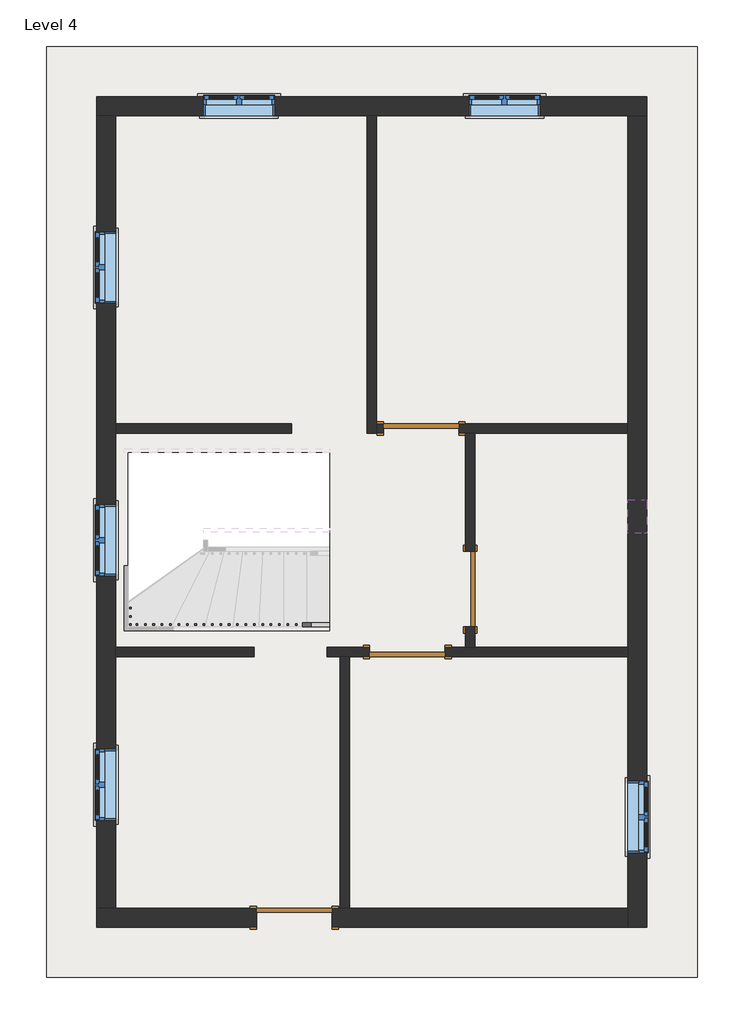
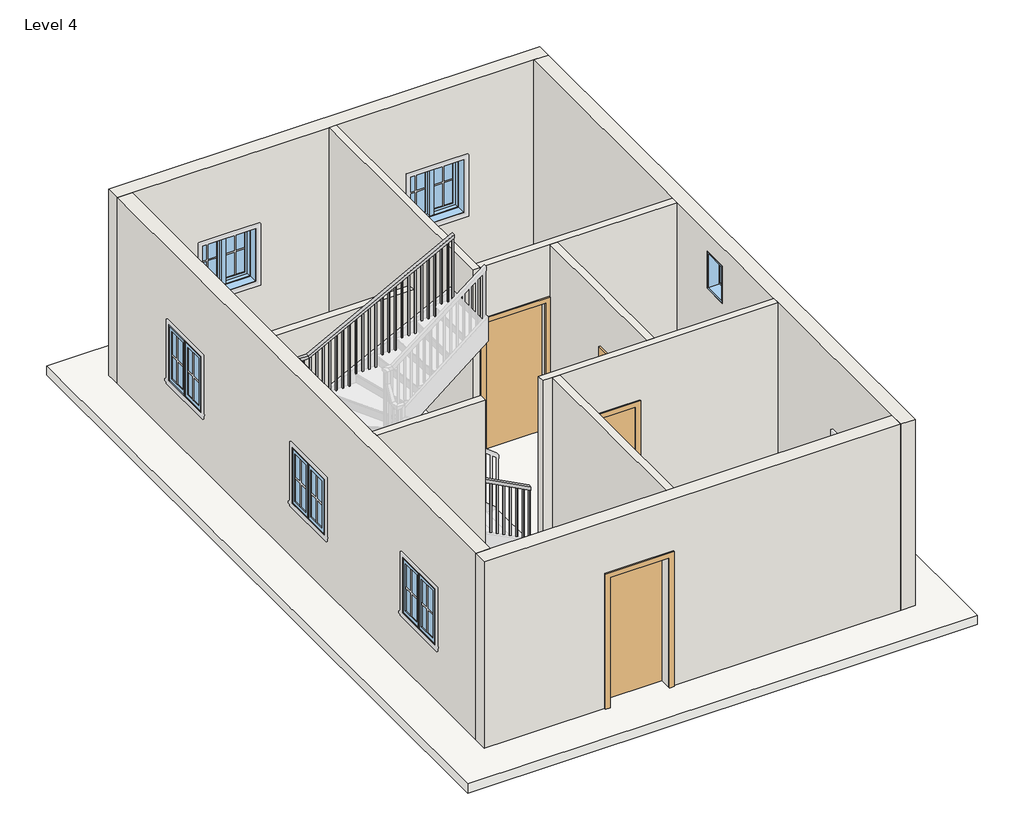
# One storey, part 1 of 2: 11 walls, 7 windows, 4 doors, 1 railing, 1 roof.
"""IFC4 building model written with IfcOpenShell, lengths in millimetres."""

from ifc_helpers import new_model, si_unit, frame, origin, place, context, project, spatial, polyline, outline, extrude, faceted_brep, transform, mapped, element, save
from components import door_e5f9f3c4, door_305aa2a5, door_a90ba1ad, window_aa618e30, window_339605e1

model = new_model("IFC4")

# Units and contexts
model_context = context("Model", 3, world=origin())
ifc_project = project(units=[si_unit("LENGTHUNIT", "METRE", prefix="MILLI")], contexts=[model_context])

# Site, building, storey
site = spatial("IfcSite", under=ifc_project)
building = spatial("IfcBuilding", under=site)
storey = spatial("IfcBuildingStorey", under=building, Name="Level 4", Elevation=6400.8)

# Doors
placement = place(None, origin())
door_shape = door_e5f9f3c4(model_context)
element("IfcDoor", 1, ObjectType="Single-Flush : 36\" x 84\"", at=placement, inside=storey, context=model_context, shape_type="MappedRepresentation", body=[
    mapped(door_shape, transform((-78.9949167, -802.9070853, 6400.8), x_axis=(0.0, -1.0, 0.0), y_axis=(1.0, 0.0, 0.0), z_axis=(0.0, 0.0, 1.0))),
])
element("IfcDoor", 2, ObjectType="Single-Flush : 36\" x 84\"", at=placement, inside=storey, context=model_context, shape_type="MappedRepresentation", body=[
    mapped(door_shape, transform((-840.9949167, -1564.9070853, 6400.8), x_axis=(-1.0, 0.0, 0.0), y_axis=(0.0, -1.0, 0.0), z_axis=(0.0, 0.0, 1.0))),
])
door_2_shape = door_305aa2a5(model_context)
element("IfcDoor", 3, ObjectType="Single-Flush : 36\" x 84\"", at=placement, inside=storey, context=model_context, shape_type="MappedRepresentation", body=[
    mapped(door_2_shape, transform((-675.8949167, 1140.1929147, 6400.8), x_axis=(-1.0, 0.0, 0.0), y_axis=(0.0, -1.0, 0.0), z_axis=(0.0, 0.0, 1.0))),
])
door_3_shape = door_a90ba1ad(model_context)
element("IfcDoor", 4, ObjectType="Single-Flush : 36\" x 84\"", at=placement, inside=storey, context=model_context, shape_type="MappedRepresentation", body=[
    mapped(door_3_shape, transform((-2212.5949167, -4784.3570853, 6400.8), x_axis=(-1.0, 0.0, 0.0), y_axis=(0.0, -1.0, 0.0), z_axis=(0.0, 0.0, 1.0))),
])

# Railing
element("IfcRailing", 5, ObjectType="Handrail - Rectangular", at=placement, inside=storey, context=model_context, shape_type="SolidModel", body=[
    faceted_brep([(-1783.4132248, -1260.1070853, 7484.5333333), (-1783.4132248, -1260.1070853, 7427.0742652), (-1783.4132248, -1209.3070853, 7427.0742652), (-1783.4132248, -1209.3070853, 7484.5333333), (-4041.1382869, -1260.1070853, 8677.8239201), (-4053.7373514, -1260.1070853, 8627.0239201), (-4053.7373514, -1209.3070853, 8627.0239201), (-4041.1382869, -1209.3070853, 8677.8239201), (-4225.5449167, -1260.1070853, 8677.8239201), (-4225.5449167, -1260.1070853, 8627.0239201), (-4174.7449167, -1209.3070853, 8627.0239201), (-4174.7449167, -1209.3070853, 8677.8239201), (-4225.5449167, -972.7952032, 8677.8239201), (-4225.5449167, -964.8446271, 8627.0239201), (-4174.7449167, -964.8446271, 8627.0239201), (-4174.7449167, -972.7952032, 8677.8239201), (-4225.5449167, 560.7810325, 9169.9094132), (-4225.5449167, 568.7316087, 9119.1094132), (-4174.7449167, 568.7316087, 9119.1094132), (-4174.7449167, 560.7810325, 9169.9094132), (-4225.5449167, 848.0929147, 9169.9094132), (-4225.5449167, 848.0929147, 9119.1094132), (-4174.7449167, 797.2929147, 9119.1094132), (-4174.7449167, 797.2929147, 9169.9094132), (-4041.1382869, 848.0929147, 9169.9094132), (-4028.5392223, 848.0929147, 9119.1094132), (-4028.5392223, 797.2929147, 9119.1094132), (-4041.1382869, 797.2929147, 9169.9094132), (-1783.4132248, 848.0929147, 10363.2), (-1783.4132248, 797.2929147, 10363.2), (-1783.4132248, 797.2929147, 10305.7409318), (-1783.4132248, 848.0929147, 10305.7409318)], [[[0, 1, 2, 3]], [[1, 0, 4, 5]], [[2, 1, 5, 6]], [[3, 2, 6, 7]], [[0, 3, 7, 4]], [[5, 4, 8, 9]], [[6, 5, 9, 10]], [[7, 6, 10, 11]], [[4, 7, 11, 8]], [[9, 8, 12, 13]], [[10, 9, 13, 14]], [[11, 10, 14, 15]], [[8, 11, 15, 12]], [[13, 12, 16, 17]], [[14, 13, 17, 18]], [[15, 14, 18, 19]], [[12, 15, 19, 16]], [[17, 16, 20, 21]], [[18, 17, 21, 22]], [[19, 18, 22, 23]], [[16, 19, 23, 20]], [[21, 20, 24, 25]], [[22, 21, 25, 26]], [[23, 22, 26, 27]], [[20, 23, 27, 24]], [[28, 29, 30, 31]], [[25, 24, 28, 31]], [[26, 25, 31, 30]], [[27, 26, 30, 29]], [[24, 27, 29, 28]]]),
    extrude(outline(polyline([(10258.4597858, -1872.8699167), (9279.4666667, -1872.8699167), (9279.4666667, -1853.8199167), (10268.5284102, -1853.8199167), (10258.4597858, -1872.8699167)])), frame((0.0, 813.1679147, 0.0), z_axis=(0.0, 1.0, 0.0), x_axis=(0.0, 0.0, 1.0)), (0.0, 0.0, 1.0), 19.05),
    extrude(outline(polyline([(10204.7604556, -1974.4699167), (9279.4666667, -1974.4699167), (9279.4666667, -1955.4199167), (10214.82908, -1955.4199167), (10204.7604556, -1974.4699167)])), frame((0.0, 813.1679147, 0.0), z_axis=(0.0, 1.0, 0.0), x_axis=(0.0, 0.0, 1.0)), (0.0, 0.0, 1.0), 19.05),
    extrude(outline(polyline([(10151.0611254, -2076.0699167), (9110.1333333, -2076.0699167), (9110.1333333, -2057.0199167), (10161.1297498, -2057.0199167), (10151.0611254, -2076.0699167)])), frame((0.0, 813.1679147, 0.0), z_axis=(0.0, 1.0, 0.0), x_axis=(0.0, 0.0, 1.0)), (0.0, 0.0, 1.0), 19.05),
    extrude(outline(polyline([(10097.3617952, -2177.6699167), (9110.1333333, -2177.6699167), (9110.1333333, -2158.6199167), (10107.4304196, -2158.6199167), (10097.3617952, -2177.6699167)])), frame((0.0, 813.1679147, 0.0), z_axis=(0.0, 1.0, 0.0), x_axis=(0.0, 0.0, 1.0)), (0.0, 0.0, 1.0), 19.05),
    extrude(outline(polyline([(10043.662465, -2279.2699167), (9110.1333333, -2279.2699167), (9110.1333333, -2260.2199167), (10053.7310894, -2260.2199167), (10043.662465, -2279.2699167)])), frame((0.0, 813.1679147, 0.0), z_axis=(0.0, 1.0, 0.0), x_axis=(0.0, 0.0, 1.0)), (0.0, 0.0, 1.0), 19.05),
    extrude(outline(polyline([(9989.9631348, -2380.8699167), (8940.8, -2380.8699167), (8940.8, -2361.8199167), (10000.0317592, -2361.8199167), (9989.9631348, -2380.8699167)])), frame((0.0, 813.1679147, 0.0), z_axis=(0.0, 1.0, 0.0), x_axis=(0.0, 0.0, 1.0)), (0.0, 0.0, 1.0), 19.05),
    extrude(outline(polyline([(9936.2638046, -2482.4699167), (8940.8, -2482.4699167), (8940.8, -2463.4199167), (9946.332429, -2463.4199167), (9936.2638046, -2482.4699167)])), frame((0.0, 813.1679147, 0.0), z_axis=(0.0, 1.0, 0.0), x_axis=(0.0, 0.0, 1.0)), (0.0, 0.0, 1.0), 19.05),
    extrude(outline(polyline([(9882.5644744, -2584.0699167), (8940.8, -2584.0699167), (8940.8, -2565.0199167), (9892.6330988, -2565.0199167), (9882.5644744, -2584.0699167)])), frame((0.0, 813.1679147, 0.0), z_axis=(0.0, 1.0, 0.0), x_axis=(0.0, 0.0, 1.0)), (0.0, 0.0, 1.0), 19.05),
    extrude(outline(polyline([(9828.8651442, -2685.6699167), (8771.4666667, -2685.6699167), (8771.4666667, -2666.6199167), (9838.9337686, -2666.6199167), (9828.8651442, -2685.6699167)])), frame((0.0, 813.1679147, 0.0), z_axis=(0.0, 1.0, 0.0), x_axis=(0.0, 0.0, 1.0)), (0.0, 0.0, 1.0), 19.05),
    extrude(outline(polyline([(9775.165814, -2787.2699167), (8771.4666667, -2787.2699167), (8771.4666667, -2768.2199167), (9785.2344384, -2768.2199167), (9775.165814, -2787.2699167)])), frame((0.0, 813.1679147, 0.0), z_axis=(0.0, 1.0, 0.0), x_axis=(0.0, 0.0, 1.0)), (0.0, 0.0, 1.0), 19.05),
    extrude(outline(polyline([(9721.4664838, -2888.8699167), (8771.4666667, -2888.8699167), (8771.4666667, -2869.8199167), (9731.5351082, -2869.8199167), (9721.4664838, -2888.8699167)])), frame((0.0, 813.1679147, 0.0), z_axis=(0.0, 1.0, 0.0), x_axis=(0.0, 0.0, 1.0)), (0.0, 0.0, 1.0), 19.05),
    extrude(outline(polyline([(9667.7671536, -2990.4699167), (8602.1333333, -2990.4699167), (8602.1333333, -2971.4199167), (9677.835778, -2971.4199167), (9667.7671536, -2990.4699167)])), frame((0.0, 813.1679147, 0.0), z_axis=(0.0, 1.0, 0.0), x_axis=(0.0, 0.0, 1.0)), (0.0, 0.0, 1.0), 19.05),
    extrude(outline(polyline([(9614.0678234, -3092.0699167), (8602.1333333, -3092.0699167), (8602.1333333, -3073.0199167), (9624.1364478, -3073.0199167), (9614.0678234, -3092.0699167)])), frame((0.0, 813.1679147, 0.0), z_axis=(0.0, 1.0, 0.0), x_axis=(0.0, 0.0, 1.0)), (0.0, 0.0, 1.0), 19.05),
    extrude(outline(polyline([(9560.3684932, -3193.6699167), (8602.1333333, -3193.6699167), (8602.1333333, -3174.6199167), (9570.4371176, -3174.6199167), (9560.3684932, -3193.6699167)])), frame((0.0, 813.1679147, 0.0), z_axis=(0.0, 1.0, 0.0), x_axis=(0.0, 0.0, 1.0)), (0.0, 0.0, 1.0), 19.05),
    extrude(outline(polyline([(9506.669163, -3295.2699167), (8602.1333333, -3295.2699167), (8602.1333333, -3276.2199167), (9516.7377874, -3276.2199167), (9506.669163, -3295.2699167)])), frame((0.0, 813.1679147, 0.0), z_axis=(0.0, 1.0, 0.0), x_axis=(0.0, 0.0, 1.0)), (0.0, 0.0, 1.0), 19.05),
    extrude(outline(polyline([(9452.9698328, -3396.8699167), (8432.8, -3396.8699167), (8432.8, -3377.8199167), (9463.0384572, -3377.8199167), (9452.9698328, -3396.8699167)])), frame((0.0, 813.1679147, 0.0), z_axis=(0.0, 1.0, 0.0), x_axis=(0.0, 0.0, 1.0)), (0.0, 0.0, 1.0), 19.05),
    extrude(outline(polyline([(9399.2705026, -3498.4699167), (8432.8, -3498.4699167), (8432.8, -3479.4199167), (9409.339127, -3479.4199167), (9399.2705026, -3498.4699167)])), frame((0.0, 813.1679147, 0.0), z_axis=(0.0, 1.0, 0.0), x_axis=(0.0, 0.0, 1.0)), (0.0, 0.0, 1.0), 19.05),
    extrude(outline(polyline([(9345.5711724, -3600.0699167), (8432.8, -3600.0699167), (8432.8, -3581.0199167), (9355.6397968, -3581.0199167), (9345.5711724, -3600.0699167)])), frame((0.0, 813.1679147, 0.0), z_axis=(0.0, 1.0, 0.0), x_axis=(0.0, 0.0, 1.0)), (0.0, 0.0, 1.0), 19.05),
    extrude(outline(polyline([(9291.8718422, -3701.6699167), (8432.8, -3701.6699167), (8432.8, -3682.6199167), (9301.9404666, -3682.6199167), (9291.8718422, -3701.6699167)])), frame((0.0, 813.1679147, 0.0), z_axis=(0.0, 1.0, 0.0), x_axis=(0.0, 0.0, 1.0)), (0.0, 0.0, 1.0), 19.05),
    extrude(outline(polyline([(9238.172512, -3803.2699167), (8263.4666667, -3803.2699167), (8263.4666667, -3784.2199167), (9248.2411364, -3784.2199167), (9238.172512, -3803.2699167)])), frame((0.0, 813.1679147, 0.0), z_axis=(0.0, 1.0, 0.0), x_axis=(0.0, 0.0, 1.0)), (0.0, 0.0, 1.0), 19.05),
    extrude(outline(polyline([(9184.4731818, -3904.8699167), (8263.4666667, -3904.8699167), (8263.4666667, -3885.8199167), (9194.5418062, -3885.8199167), (9184.4731818, -3904.8699167)])), frame((0.0, 813.1679147, 0.0), z_axis=(0.0, 1.0, 0.0), x_axis=(0.0, 0.0, 1.0)), (0.0, 0.0, 1.0), 19.05),
    extrude(outline(polyline([(9130.7738516, -4006.4699167), (8263.4666667, -4006.4699167), (8263.4666667, -3987.4199167), (9140.842476, -3987.4199167), (9130.7738516, -4006.4699167)])), frame((0.0, 813.1679147, 0.0), z_axis=(0.0, 1.0, 0.0), x_axis=(0.0, 0.0, 1.0)), (0.0, 0.0, 1.0), 19.05),
    extrude(outline(polyline([(-4108.0699167, 832.2179147), (-4089.0199167, 832.2179147), (-4089.0199167, 813.1679147), (-4108.0699167, 813.1679147), (-4108.0699167, 832.2179147)])), frame((0.0, 0.0, 8263.4666667), z_axis=(0.0, 0.0, 1.0), x_axis=(1.0, 0.0, 0.0)), (0.0, 0.0, 1.0), 855.6427466),
    extrude(outline(polyline([(-4209.6699167, 787.7679147), (-4209.6699167, 806.8179147), (-4190.6199167, 806.8179147), (-4190.6199167, 787.7679147), (-4209.6699167, 787.7679147)])), frame((0.0, 0.0, 8263.4666667), z_axis=(0.0, 0.0, 1.0), x_axis=(1.0, 0.0, 0.0)), (0.0, 0.0, 1.0), 855.6427466),
    extrude(outline(polyline([(-4209.6699167, 686.1679147), (-4209.6699167, 705.2179147), (-4190.6199167, 705.2179147), (-4190.6199167, 686.1679147), (-4209.6699167, 686.1679147)])), frame((0.0, 0.0, 8263.4666667), z_axis=(0.0, 0.0, 1.0), x_axis=(1.0, 0.0, 0.0)), (0.0, 0.0, 1.0), 855.6427466),
    extrude(outline(polyline([(-4209.6699167, 584.5679147), (-4209.6699167, 603.6179147), (-4190.6199167, 603.6179147), (-4190.6199167, 584.5679147), (-4209.6699167, 584.5679147)])), frame((0.0, 0.0, 8263.4666667), z_axis=(0.0, 0.0, 1.0), x_axis=(1.0, 0.0, 0.0)), (0.0, 0.0, 1.0), 855.6427466),
    extrude(outline(polyline([(502.0179147, 9097.7026907), (502.0179147, 8094.1333333), (482.9679147, 8094.1333333), (482.9679147, 9091.5900316), (502.0179147, 9097.7026907)])), frame((-4209.6699167, 0.0, 0.0), z_axis=(1.0, 0.0, 0.0), x_axis=(0.0, 1.0, 0.0)), (0.0, 0.0, 1.0), 19.05),
    extrude(outline(polyline([(400.4179147, 9065.1018425), (400.4179147, 8094.1333333), (381.3679147, 8094.1333333), (381.3679147, 9058.9891834), (400.4179147, 9065.1018425)])), frame((-4209.6699167, 0.0, 0.0), z_axis=(1.0, 0.0, 0.0), x_axis=(0.0, 1.0, 0.0)), (0.0, 0.0, 1.0), 19.05),
    extrude(outline(polyline([(298.8179147, 9032.5009942), (298.8179147, 8094.1333333), (279.7679147, 8094.1333333), (279.7679147, 9026.3883352), (298.8179147, 9032.5009942)])), frame((-4209.6699167, 0.0, 0.0), z_axis=(1.0, 0.0, 0.0), x_axis=(0.0, 1.0, 0.0)), (0.0, 0.0, 1.0), 19.05),
    extrude(outline(polyline([(197.2179147, 8999.900146), (197.2179147, 8094.1333333), (178.1679147, 8094.1333333), (178.1679147, 8993.787487), (197.2179147, 8999.900146)])), frame((-4209.6699167, 0.0, 0.0), z_axis=(1.0, 0.0, 0.0), x_axis=(0.0, 1.0, 0.0)), (0.0, 0.0, 1.0), 19.05),
    extrude(outline(polyline([(95.6179147, 8967.2992978), (95.6179147, 8094.1333333), (76.5679147, 8094.1333333), (76.5679147, 8961.1866387), (95.6179147, 8967.2992978)])), frame((-4209.6699167, 0.0, 0.0), z_axis=(1.0, 0.0, 0.0), x_axis=(0.0, 1.0, 0.0)), (0.0, 0.0, 1.0), 19.05),
    extrude(outline(polyline([(-5.9820853, 8934.6984495), (-5.9820853, 7924.8), (-25.0320853, 7924.8), (-25.0320853, 8928.5857905), (-5.9820853, 8934.6984495)])), frame((-4209.6699167, 0.0, 0.0), z_axis=(1.0, 0.0, 0.0), x_axis=(0.0, 1.0, 0.0)), (0.0, 0.0, 1.0), 19.05),
    extrude(outline(polyline([(-107.5820853, 8902.0976013), (-107.5820853, 7924.8), (-126.6320853, 7924.8), (-126.6320853, 8895.9849423), (-107.5820853, 8902.0976013)])), frame((-4209.6699167, 0.0, 0.0), z_axis=(1.0, 0.0, 0.0), x_axis=(0.0, 1.0, 0.0)), (0.0, 0.0, 1.0), 19.05),
    extrude(outline(polyline([(-209.1820853, 8869.4967531), (-209.1820853, 7924.8), (-228.2320853, 7924.8), (-228.2320853, 8863.384094), (-209.1820853, 8869.4967531)])), frame((-4209.6699167, 0.0, 0.0), z_axis=(1.0, 0.0, 0.0), x_axis=(0.0, 1.0, 0.0)), (0.0, 0.0, 1.0), 19.05),
    extrude(outline(polyline([(-310.7820853, 8836.8959049), (-310.7820853, 7924.8), (-329.8320853, 7924.8), (-329.8320853, 8830.7832458), (-310.7820853, 8836.8959049)])), frame((-4209.6699167, 0.0, 0.0), z_axis=(1.0, 0.0, 0.0), x_axis=(0.0, 1.0, 0.0)), (0.0, 0.0, 1.0), 19.05),
    extrude(outline(polyline([(-412.3820853, 8804.2950566), (-412.3820853, 7924.8), (-431.4320853, 7924.8), (-431.4320853, 8798.1823976), (-412.3820853, 8804.2950566)])), frame((-4209.6699167, 0.0, 0.0), z_axis=(1.0, 0.0, 0.0), x_axis=(0.0, 1.0, 0.0)), (0.0, 0.0, 1.0), 19.05),
    extrude(outline(polyline([(-513.9820853, 8771.6942084), (-513.9820853, 7755.4666667), (-533.0320853, 7755.4666667), (-533.0320853, 8765.5815494), (-513.9820853, 8771.6942084)])), frame((-4209.6699167, 0.0, 0.0), z_axis=(1.0, 0.0, 0.0), x_axis=(0.0, 1.0, 0.0)), (0.0, 0.0, 1.0), 19.05),
    extrude(outline(polyline([(-615.5820853, 8739.0933602), (-615.5820853, 7755.4666667), (-634.6320853, 7755.4666667), (-634.6320853, 8732.9807011), (-615.5820853, 8739.0933602)])), frame((-4209.6699167, 0.0, 0.0), z_axis=(1.0, 0.0, 0.0), x_axis=(0.0, 1.0, 0.0)), (0.0, 0.0, 1.0), 19.05),
    extrude(outline(polyline([(-717.1820853, 8706.492512), (-717.1820853, 7755.4666667), (-736.2320853, 7755.4666667), (-736.2320853, 8700.3798529), (-717.1820853, 8706.492512)])), frame((-4209.6699167, 0.0, 0.0), z_axis=(1.0, 0.0, 0.0), x_axis=(0.0, 1.0, 0.0)), (0.0, 0.0, 1.0), 19.05),
    extrude(outline(polyline([(-818.7820853, 8673.8916637), (-818.7820853, 7755.4666667), (-837.8320853, 7755.4666667), (-837.8320853, 8667.7790047), (-818.7820853, 8673.8916637)])), frame((-4209.6699167, 0.0, 0.0), z_axis=(1.0, 0.0, 0.0), x_axis=(0.0, 1.0, 0.0)), (0.0, 0.0, 1.0), 19.05),
    extrude(outline(polyline([(-920.3820853, 8641.2908155), (-920.3820853, 7755.4666667), (-939.4320853, 7755.4666667), (-939.4320853, 8635.1781565), (-920.3820853, 8641.2908155)])), frame((-4209.6699167, 0.0, 0.0), z_axis=(1.0, 0.0, 0.0), x_axis=(0.0, 1.0, 0.0)), (0.0, 0.0, 1.0), 19.05),
    extrude(outline(polyline([(-4209.6699167, -1041.0320853), (-4209.6699167, -1021.9820853), (-4190.6199167, -1021.9820853), (-4190.6199167, -1041.0320853), (-4209.6699167, -1041.0320853)])), frame((0.0, 0.0, 7586.1333333), z_axis=(0.0, 0.0, 1.0), x_axis=(1.0, 0.0, 0.0)), (0.0, 0.0, 1.0), 1040.8905868),
    extrude(outline(polyline([(-4209.6699167, -1142.6320853), (-4209.6699167, -1123.5820853), (-4190.6199167, -1123.5820853), (-4190.6199167, -1142.6320853), (-4209.6699167, -1142.6320853)])), frame((0.0, 0.0, 7586.1333333), z_axis=(0.0, 0.0, 1.0), x_axis=(1.0, 0.0, 0.0)), (0.0, 0.0, 1.0), 1040.8905868),
    extrude(outline(polyline([(-4110.6882248, -1244.2320853), (-4129.7382248, -1244.2320853), (-4129.7382248, -1225.1820853), (-4110.6882248, -1225.1820853), (-4110.6882248, -1244.2320853)])), frame((0.0, 0.0, 7586.1333333), z_axis=(0.0, 0.0, 1.0), x_axis=(1.0, 0.0, 0.0)), (0.0, 0.0, 1.0), 1040.8905868),
    extrude(outline(polyline([(8613.4938418, -4028.1382248), (7586.1333333, -4028.1382248), (7586.1333333, -4009.0882248), (8603.4252174, -4009.0882248), (8613.4938418, -4028.1382248)])), frame((0.0, -1244.2320853, 0.0), z_axis=(0.0, 1.0, 0.0), x_axis=(0.0, 0.0, 1.0)), (0.0, 0.0, 1.0), 19.05),
    extrude(outline(polyline([(8559.7945116, -3926.5382248), (7586.1333333, -3926.5382248), (7586.1333333, -3907.4882248), (8549.7258872, -3907.4882248), (8559.7945116, -3926.5382248)])), frame((0.0, -1244.2320853, 0.0), z_axis=(0.0, 1.0, 0.0), x_axis=(0.0, 0.0, 1.0)), (0.0, 0.0, 1.0), 19.05),
    extrude(outline(polyline([(8506.0951814, -3824.9382248), (7586.1333333, -3824.9382248), (7586.1333333, -3805.8882248), (8496.026557, -3805.8882248), (8506.0951814, -3824.9382248)])), frame((0.0, -1244.2320853, 0.0), z_axis=(0.0, 1.0, 0.0), x_axis=(0.0, 0.0, 1.0)), (0.0, 0.0, 1.0), 19.05),
    extrude(outline(polyline([(8452.3958512, -3723.3382248), (7586.1333333, -3723.3382248), (7586.1333333, -3704.2882248), (8442.3272268, -3704.2882248), (8452.3958512, -3723.3382248)])), frame((0.0, -1244.2320853, 0.0), z_axis=(0.0, 1.0, 0.0), x_axis=(0.0, 0.0, 1.0)), (0.0, 0.0, 1.0), 19.05),
    extrude(outline(polyline([(8398.696521, -3621.7382248), (7416.8, -3621.7382248), (7416.8, -3602.6882248), (8388.6278966, -3602.6882248), (8398.696521, -3621.7382248)])), frame((0.0, -1244.2320853, 0.0), z_axis=(0.0, 1.0, 0.0), x_axis=(0.0, 0.0, 1.0)), (0.0, 0.0, 1.0), 19.05),
    extrude(outline(polyline([(8344.9971908, -3520.1382248), (7416.8, -3520.1382248), (7416.8, -3501.0882248), (8334.9285664, -3501.0882248), (8344.9971908, -3520.1382248)])), frame((0.0, -1244.2320853, 0.0), z_axis=(0.0, 1.0, 0.0), x_axis=(0.0, 0.0, 1.0)), (0.0, 0.0, 1.0), 19.05),
    extrude(outline(polyline([(8291.2978606, -3418.5382248), (7416.8, -3418.5382248), (7416.8, -3399.4882248), (8281.2292362, -3399.4882248), (8291.2978606, -3418.5382248)])), frame((0.0, -1244.2320853, 0.0), z_axis=(0.0, 1.0, 0.0), x_axis=(0.0, 0.0, 1.0)), (0.0, 0.0, 1.0), 19.05),
    extrude(outline(polyline([(8237.5985304, -3316.9382248), (7416.8, -3316.9382248), (7416.8, -3297.8882248), (8227.529906, -3297.8882248), (8237.5985304, -3316.9382248)])), frame((0.0, -1244.2320853, 0.0), z_axis=(0.0, 1.0, 0.0), x_axis=(0.0, 0.0, 1.0)), (0.0, 0.0, 1.0), 19.05),
    extrude(outline(polyline([(8183.8992002, -3215.3382248), (7247.4666667, -3215.3382248), (7247.4666667, -3196.2882248), (8173.8305758, -3196.2882248), (8183.8992002, -3215.3382248)])), frame((0.0, -1244.2320853, 0.0), z_axis=(0.0, 1.0, 0.0), x_axis=(0.0, 0.0, 1.0)), (0.0, 0.0, 1.0), 19.05),
    extrude(outline(polyline([(8130.19987, -3113.7382248), (7247.4666667, -3113.7382248), (7247.4666667, -3094.6882248), (8120.1312456, -3094.6882248), (8130.19987, -3113.7382248)])), frame((0.0, -1244.2320853, 0.0), z_axis=(0.0, 1.0, 0.0), x_axis=(0.0, 0.0, 1.0)), (0.0, 0.0, 1.0), 19.05),
    extrude(outline(polyline([(8076.5005398, -3012.1382248), (7247.4666667, -3012.1382248), (7247.4666667, -2993.0882248), (8066.4319154, -2993.0882248), (8076.5005398, -3012.1382248)])), frame((0.0, -1244.2320853, 0.0), z_axis=(0.0, 1.0, 0.0), x_axis=(0.0, 0.0, 1.0)), (0.0, 0.0, 1.0), 19.05),
    extrude(outline(polyline([(8022.8012096, -2910.5382248), (7078.1333333, -2910.5382248), (7078.1333333, -2891.4882248), (8012.7325852, -2891.4882248), (8022.8012096, -2910.5382248)])), frame((0.0, -1244.2320853, 0.0), z_axis=(0.0, 1.0, 0.0), x_axis=(0.0, 0.0, 1.0)), (0.0, 0.0, 1.0), 19.05),
    extrude(outline(polyline([(7969.1018794, -2808.9382248), (7078.1333333, -2808.9382248), (7078.1333333, -2789.8882248), (7959.033255, -2789.8882248), (7969.1018794, -2808.9382248)])), frame((0.0, -1244.2320853, 0.0), z_axis=(0.0, 1.0, 0.0), x_axis=(0.0, 0.0, 1.0)), (0.0, 0.0, 1.0), 19.05),
    extrude(outline(polyline([(7915.4025492, -2707.3382248), (7078.1333333, -2707.3382248), (7078.1333333, -2688.2882248), (7905.3339248, -2688.2882248), (7915.4025492, -2707.3382248)])), frame((0.0, -1244.2320853, 0.0), z_axis=(0.0, 1.0, 0.0), x_axis=(0.0, 0.0, 1.0)), (0.0, 0.0, 1.0), 19.05),
    extrude(outline(polyline([(7861.703219, -2605.7382248), (6908.8, -2605.7382248), (6908.8, -2586.6882248), (7851.6345946, -2586.6882248), (7861.703219, -2605.7382248)])), frame((0.0, -1244.2320853, 0.0), z_axis=(0.0, 1.0, 0.0), x_axis=(0.0, 0.0, 1.0)), (0.0, 0.0, 1.0), 19.05),
    extrude(outline(polyline([(7808.0038888, -2504.1382248), (6908.8, -2504.1382248), (6908.8, -2485.0882248), (7797.9352644, -2485.0882248), (7808.0038888, -2504.1382248)])), frame((0.0, -1244.2320853, 0.0), z_axis=(0.0, 1.0, 0.0), x_axis=(0.0, 0.0, 1.0)), (0.0, 0.0, 1.0), 19.05),
    extrude(outline(polyline([(7754.3045586, -2402.5382248), (6908.8, -2402.5382248), (6908.8, -2383.4882248), (7744.2359342, -2383.4882248), (7754.3045586, -2402.5382248)])), frame((0.0, -1244.2320853, 0.0), z_axis=(0.0, 1.0, 0.0), x_axis=(0.0, 0.0, 1.0)), (0.0, 0.0, 1.0), 19.05),
    extrude(outline(polyline([(7700.6052284, -2300.9382248), (6739.4666667, -2300.9382248), (6739.4666667, -2281.8882248), (7690.536604, -2281.8882248), (7700.6052284, -2300.9382248)])), frame((0.0, -1244.2320853, 0.0), z_axis=(0.0, 1.0, 0.0), x_axis=(0.0, 0.0, 1.0)), (0.0, 0.0, 1.0), 19.05),
    extrude(outline(polyline([(7646.9058982, -2199.3382248), (6739.4666667, -2199.3382248), (6739.4666667, -2180.2882248), (7636.8372738, -2180.2882248), (7646.9058982, -2199.3382248)])), frame((0.0, -1244.2320853, 0.0), z_axis=(0.0, 1.0, 0.0), x_axis=(0.0, 0.0, 1.0)), (0.0, 0.0, 1.0), 19.05),
    extrude(outline(polyline([(7593.206568, -2097.7382248), (6739.4666667, -2097.7382248), (6739.4666667, -2078.6882248), (7583.1379436, -2078.6882248), (7593.206568, -2097.7382248)])), frame((0.0, -1244.2320853, 0.0), z_axis=(0.0, 1.0, 0.0), x_axis=(0.0, 0.0, 1.0)), (0.0, 0.0, 1.0), 19.05),
    extrude(outline(polyline([(7539.5072378, -1996.1382248), (6570.1333333, -1996.1382248), (6570.1333333, -1977.0882248), (7529.4386134, -1977.0882248), (7539.5072378, -1996.1382248)])), frame((0.0, -1244.2320853, 0.0), z_axis=(0.0, 1.0, 0.0), x_axis=(0.0, 0.0, 1.0)), (0.0, 0.0, 1.0), 19.05),
    extrude(outline(polyline([(7485.8079076, -1894.5382248), (6570.1333333, -1894.5382248), (6570.1333333, -1875.4882248), (7475.7392831, -1875.4882248), (7485.8079076, -1894.5382248)])), frame((0.0, -1244.2320853, 0.0), z_axis=(0.0, 1.0, 0.0), x_axis=(0.0, 0.0, 1.0)), (0.0, 0.0, 1.0), 19.05),
    extrude(outline(polyline([(-4209.6699167, 813.1679147), (-4209.6699167, 832.2179147), (-4190.6199167, 832.2179147), (-4190.6199167, 813.1679147), (-4209.6699167, 813.1679147)])), frame((0.0, 0.0, 8263.4666667), z_axis=(0.0, 0.0, 1.0), x_axis=(1.0, 0.0, 0.0)), (0.0, 0.0, 1.0), 855.6427466),
    extrude(outline(polyline([(-4190.6199167, -1244.2320853), (-4209.6699167, -1244.2320853), (-4209.6699167, -1225.1820853), (-4190.6199167, -1225.1820853), (-4190.6199167, -1244.2320853)])), frame((0.0, 0.0, 7586.1333333), z_axis=(0.0, 0.0, 1.0), x_axis=(1.0, 0.0, 0.0)), (0.0, 0.0, 1.0), 1040.8905868),
    extrude(outline(polyline([(10295.6723074, -1802.4632248), (9279.4666667, -1802.4632248), (9279.4666667, -1783.4132248), (10305.7409318, -1783.4132248), (10295.6723074, -1802.4632248)])), frame((0.0, 813.1679147, 0.0), z_axis=(0.0, 1.0, 0.0), x_axis=(0.0, 0.0, 1.0)), (0.0, 0.0, 1.0), 19.05),
    extrude(outline(polyline([(7437.1428896, -1802.4632248), (6570.1333333, -1802.4632248), (6570.1333333, -1783.4132248), (7427.0742652, -1783.4132248), (7437.1428896, -1802.4632248)])), frame((0.0, -1244.2320853, 0.0), z_axis=(0.0, 1.0, 0.0), x_axis=(0.0, 0.0, 1.0)), (0.0, 0.0, 1.0), 19.05),
])

# Roof
element("IfcRoof", 6, ObjectType="Generic - 12\"", at=placement, inside=storey, context=model_context, shape_type="SweptSolid", body=[
    extrude(outline(polyline([(-5216.1449167, -5508.2570853), (-5216.1449167, 5769.3429147), (2670.5550833, 5769.3429147), (2670.5550833, -5508.2570853), (-5216.1449167, -5508.2570853)]), holes=[polyline([(-1783.4132248, 848.0929147), (-4225.5449167, 848.0929147), (-4225.5449167, -1209.3070853), (-1783.4132248, -1209.3070853), (-1783.4132248, 848.0929147)])]), frame((0.0, 0.0, 6248.4), z_axis=(0.0, 0.0, 1.0), x_axis=(1.0, 0.0, 0.0)), (0.0, 0.0, 1.0), 152.4),
])

# Walls
element("IfcWall", 7, ObjectType="WALL4.5\"", at=placement, inside=storey, context=model_context, shape_type="Brep", body=[
    faceted_brep([(-1329.9449167, 4931.1429147, 6400.8), (-1329.9449167, 1083.0429147, 6400.8), (-1329.9449167, 1083.0429147, 9448.8), (-1329.9449167, 4931.1429147, 9448.8), (-1215.6449167, 4931.1429147, 6400.8), (-1215.6449167, 4931.1429147, 9448.8), (-1215.6449167, 1197.3429147, 9448.8), (-1215.6449167, 1083.0429147, 9448.8), (-1215.6449167, 1083.0429147, 6400.8), (-1215.6449167, 1197.3429147, 6400.8)], [[[0, 1, 2, 3]], [[4, 5, 6, 7, 8, 9]], [[1, 0, 4, 9, 8]], [[0, 3, 5, 4]], [[2, 1, 8, 7]], [[3, 2, 7, 6, 5]]]),
])
element("IfcWall", 8, ObjectType="WALL4.5\"", at=placement, inside=storey, context=model_context, shape_type="Brep", body=[
    faceted_brep([(-1215.6449167, 1083.0429147, 6400.8), (-1133.0949167, 1083.0429147, 6400.8), (-1133.0949167, 1083.0429147, 8534.4), (-218.6949167, 1083.0429147, 8534.4), (-218.6949167, 1083.0429147, 6400.8), (-136.1449167, 1083.0429147, 6400.8), (-21.8449167, 1083.0429147, 6400.8), (1832.3550833, 1083.0429147, 6400.8), (1832.3550833, 1083.0429147, 9448.8), (-21.8449167, 1083.0429147, 9448.8), (-136.1449167, 1083.0429147, 9448.8), (-1215.6449167, 1083.0429147, 9448.8), (-1133.0949167, 1197.3429147, 8534.4), (-1133.0949167, 1197.3429147, 6400.8), (-1215.6449167, 1197.3429147, 6400.8), (-1215.6449167, 1197.3429147, 9448.8), (1832.3550833, 1197.3429147, 9448.8), (1832.3550833, 1197.3429147, 6400.8), (-218.6949167, 1197.3429147, 6400.8), (-218.6949167, 1197.3429147, 8534.4)], [[[0, 1, 2, 3, 4, 5, 6, 7, 8, 9, 10, 11]], [[12, 13, 14, 15, 16, 17, 18, 19]], [[18, 17, 7, 6, 5, 4]], [[14, 13, 1, 0]], [[0, 11, 15, 14]], [[8, 7, 17, 16]], [[2, 1, 13, 12]], [[3, 2, 12, 19]], [[4, 3, 19, 18]], [[11, 10, 9, 8, 16, 15]]]),
])
element("IfcWall", 9, ObjectType="WALL4.5\"", at=placement, inside=storey, context=model_context, shape_type="SweptSolid", body=[
    extrude(outline(polyline([(-2244.3449167, 1083.0429147), (-4377.9449167, 1083.0429147), (-4377.9449167, 1197.3429147), (-2244.3449167, 1197.3429147), (-2244.3449167, 1083.0429147)])), frame((0.0, 0.0, 6400.8), z_axis=(0.0, 0.0, 1.0), x_axis=(1.0, 0.0, 0.0)), (0.0, 0.0, 1.0), 3048.0),
])
element("IfcWall", 10, ObjectType="WALL4.5\"", at=placement, inside=storey, context=model_context, shape_type="SweptSolid", body=[
    extrude(outline(polyline([(-1260.1070853, 8534.4), (-1260.1070853, 6400.8), (-1507.7570853, 6400.8), (-1507.7570853, 9448.8), (1083.0429147, 9448.8), (1083.0429147, 6400.8), (-345.7070853, 6400.8), (-345.7070853, 8534.4), (-1260.1070853, 8534.4)])), frame((-136.1449167, 0.0, 0.0), z_axis=(1.0, 0.0, 0.0), x_axis=(0.0, 1.0, 0.0)), (0.0, 0.0, 1.0), 114.3),
])
element("IfcWall", 11, ObjectType="WALL4.5\"", at=placement, inside=storey, context=model_context, shape_type="SweptSolid", body=[
    extrude(outline(polyline([(-2701.5449167, -1622.0570853), (-4377.9449167, -1622.0570853), (-4377.9449167, -1507.7570853), (-2701.5449167, -1507.7570853), (-2701.5449167, -1622.0570853)])), frame((0.0, 0.0, 6400.8), z_axis=(0.0, 0.0, 1.0), x_axis=(1.0, 0.0, 0.0)), (0.0, 0.0, 1.0), 3048.0),
])
element("IfcWall", 12, ObjectType="WALL4.5\"", at=placement, inside=storey, context=model_context, shape_type="Brep", body=[
    faceted_brep([(-1812.5449167, -1622.0570853, 6400.8), (-1660.1449167, -1622.0570853, 6400.8), (-1545.8449167, -1622.0570853, 6400.8), (-1298.1949167, -1622.0570853, 6400.8), (-1298.1949167, -1622.0570853, 8534.4), (-383.7949167, -1622.0570853, 8534.4), (-383.7949167, -1622.0570853, 6400.8), (1832.3550833, -1622.0570853, 6400.8), (1832.3550833, -1622.0570853, 9448.8), (-1545.8449167, -1622.0570853, 9448.8), (-1660.1449167, -1622.0570853, 9448.8), (-1812.5449167, -1622.0570853, 9448.8), (-1298.1949167, -1507.7570853, 8534.4), (-1298.1949167, -1507.7570853, 6400.8), (-1812.5449167, -1507.7570853, 6400.8), (-1812.5449167, -1507.7570853, 9448.8), (-136.1449167, -1507.7570853, 9448.8), (-21.8449167, -1507.7570853, 9448.8), (1832.3550833, -1507.7570853, 9448.8), (1832.3550833, -1507.7570853, 6400.8), (-21.8449167, -1507.7570853, 6400.8), (-136.1449167, -1507.7570853, 6400.8), (-383.7949167, -1507.7570853, 6400.8), (-383.7949167, -1507.7570853, 8534.4)], [[[0, 1, 2, 3, 4, 5, 6, 7, 8, 9, 10, 11]], [[12, 13, 14, 15, 16, 17, 18, 19, 20, 21, 22, 23]], [[14, 13, 3, 2, 1, 0]], [[22, 21, 20, 19, 7, 6]], [[0, 11, 15, 14]], [[8, 7, 19, 18]], [[4, 3, 13, 12]], [[5, 4, 12, 23]], [[6, 5, 23, 22]], [[11, 10, 9, 8, 18, 17, 16, 15]]]),
])
element("IfcWall", 13, ObjectType="WALL4.5\"", at=placement, inside=storey, context=model_context, shape_type="SweptSolid", body=[
    extrude(outline(polyline([(-1660.1449167, -4670.0570853), (-1660.1449167, -1622.0570853), (-1545.8449167, -1622.0570853), (-1545.8449167, -4670.0570853), (-1660.1449167, -4670.0570853)])), frame((0.0, 0.0, 6400.8), z_axis=(0.0, 0.0, 1.0), x_axis=(1.0, 0.0, 0.0)), (0.0, 0.0, 1.0), 3048.0),
])
element("IfcWall", 14, ObjectType="WALL9\"", at=placement, inside=storey, context=model_context, shape_type="Brep", body=[
    faceted_brep([(-4606.5449167, 4931.1429147, 6400.8), (-4377.9449167, 4931.1429147, 6400.8), (-1329.9449167, 4931.1429147, 6400.8), (-1215.6449167, 4931.1429147, 6400.8), (1832.3550833, 4931.1429147, 6400.8), (2060.9550833, 4931.1429147, 6400.8), (2060.9550833, 4931.1429147, 9448.8), (1832.3550833, 4931.1429147, 9448.8), (-1215.6449167, 4931.1429147, 9448.8), (-1329.9449167, 4931.1429147, 9448.8), (-4377.9449167, 4931.1429147, 9448.8), (-4606.5449167, 4931.1429147, 9448.8), (-2450.7199167, 4931.1429147, 8229.6), (-2450.7199167, 4931.1429147, 7315.2), (-3314.3199167, 4931.1429147, 7315.2), (-3314.3199167, 4931.1429147, 8229.6), (768.7300833, 4931.1429147, 8229.6), (768.7300833, 4931.1429147, 7315.2), (-94.8699167, 4931.1429147, 7315.2), (-94.8699167, 4931.1429147, 8229.6), (-4606.5449167, 5159.7429147, 6400.8), (-4606.5449167, 5159.7429147, 9448.8), (2060.9550833, 5159.7429147, 9448.8), (2060.9550833, 5159.7429147, 6400.8), (-2450.7199167, 5159.7429147, 8229.6), (-3314.3199167, 5159.7429147, 8229.6), (-3314.3199167, 5159.7429147, 7315.2), (-2450.7199167, 5159.7429147, 7315.2), (768.7300833, 5159.7429147, 8229.6), (-94.8699167, 5159.7429147, 8229.6), (-94.8699167, 5159.7429147, 7315.2), (768.7300833, 5159.7429147, 7315.2)], [[[0, 1, 2, 3, 4, 5, 6, 7, 8, 9, 10, 11], [12, 13, 14, 15], [16, 17, 18, 19]], [[20, 21, 22, 23], [24, 25, 26, 27], [28, 29, 30, 31]], [[5, 4, 3, 2, 1, 0, 20, 23]], [[6, 5, 23, 22]], [[0, 11, 21, 20]], [[11, 10, 9, 8, 7, 6, 22, 21]], [[13, 12, 24, 27]], [[14, 13, 27, 26]], [[15, 14, 26, 25]], [[12, 15, 25, 24]], [[17, 16, 28, 31]], [[18, 17, 31, 30]], [[19, 18, 30, 29]], [[16, 19, 29, 28]]]),
])
element("IfcWall", 15, ObjectType="WALL9\"", at=placement, inside=storey, context=model_context, shape_type="Brep", body=[
    faceted_brep([(1832.3550833, 4931.1429147, 6400.8), (1832.3550833, 1197.3429147, 6400.8), (1832.3550833, 1083.0429147, 6400.8), (1832.3550833, -1507.7570853, 6400.8), (1832.3550833, -1622.0570853, 6400.8), (1832.3550833, -4670.0570853, 6400.8), (1832.3550833, -4898.6570853, 6400.8), (1832.3550833, -4898.6570853, 9448.8), (1832.3550833, -4670.0570853, 9448.8), (1832.3550833, -1622.0570853, 9448.8), (1832.3550833, -1507.7570853, 9448.8), (1832.3550833, 1083.0429147, 9448.8), (1832.3550833, 1197.3429147, 9448.8), (1832.3550833, 4931.1429147, 9448.8), (1832.3550833, -129.8070853, 9144.0), (1832.3550833, -129.8070853, 8534.4), (1832.3550833, 276.5929147, 8534.4), (1832.3550833, 276.5929147, 9144.0), (1832.3550833, -3996.9570853, 8229.6), (1832.3550833, -3996.9570853, 7315.2), (1832.3550833, -3133.3570853, 7315.2), (1832.3550833, -3133.3570853, 8229.6), (2060.9550833, 4931.1429147, 6400.8), (2060.9550833, 4931.1429147, 9448.8), (2060.9550833, -4898.6570853, 9448.8), (2060.9550833, -4898.6570853, 6400.8), (2060.9550833, -129.8070853, 9144.0), (2060.9550833, 276.5929147, 9144.0), (2060.9550833, 276.5929147, 8534.4), (2060.9550833, -129.8070853, 8534.4), (2060.9550833, -3996.9570853, 8229.6), (2060.9550833, -3133.3570853, 8229.6), (2060.9550833, -3133.3570853, 7315.2), (2060.9550833, -3996.9570853, 7315.2)], [[[0, 1, 2, 3, 4, 5, 6, 7, 8, 9, 10, 11, 12, 13], [14, 15, 16, 17], [18, 19, 20, 21]], [[22, 23, 24, 25], [26, 27, 28, 29], [30, 31, 32, 33]], [[6, 5, 4, 3, 2, 1, 0, 22, 25]], [[0, 13, 23, 22]], [[7, 6, 25, 24]], [[13, 12, 11, 10, 9, 8, 7, 24, 23]], [[15, 14, 26, 29]], [[16, 15, 29, 28]], [[17, 16, 28, 27]], [[14, 17, 27, 26]], [[19, 18, 30, 33]], [[20, 19, 33, 32]], [[21, 20, 32, 31]], [[18, 21, 31, 30]]]),
])
element("IfcWall", 16, ObjectType="WALL9\"", at=placement, inside=storey, context=model_context, shape_type="Brep", body=[
    faceted_brep([(-2669.7949167, -4670.0570853, 8534.4), (-2669.7949167, -4670.0570853, 6400.8), (-4377.9449167, -4670.0570853, 6400.8), (-4606.5449167, -4670.0570853, 6400.8), (-4606.5449167, -4670.0570853, 9448.8), (-4377.9449167, -4670.0570853, 9448.8), (-1660.1449167, -4670.0570853, 9448.8), (-1545.8449167, -4670.0570853, 9448.8), (1832.3550833, -4670.0570853, 9448.8), (1832.3550833, -4670.0570853, 6400.8), (-1545.8449167, -4670.0570853, 6400.8), (-1660.1449167, -4670.0570853, 6400.8), (-1755.3949167, -4670.0570853, 6400.8), (-1755.3949167, -4670.0570853, 8534.4), (-4606.5449167, -4898.6570853, 6400.8), (-2669.7949167, -4898.6570853, 6400.8), (-2669.7949167, -4898.6570853, 8534.4), (-1755.3949167, -4898.6570853, 8534.4), (-1755.3949167, -4898.6570853, 6400.8), (1832.3550833, -4898.6570853, 6400.8), (1832.3550833, -4898.6570853, 9448.8), (-4606.5449167, -4898.6570853, 9448.8)], [[[0, 1, 2, 3, 4, 5, 6, 7, 8, 9, 10, 11, 12, 13]], [[14, 15, 16, 17, 18, 19, 20, 21]], [[3, 2, 1, 15, 14]], [[12, 11, 10, 9, 19, 18]], [[9, 8, 20, 19]], [[4, 3, 14, 21]], [[16, 15, 1, 0]], [[17, 16, 0, 13]], [[18, 17, 13, 12]], [[8, 7, 6, 5, 4, 21, 20]]]),
])
element("IfcWall", 17, ObjectType="WALL9\"", at=placement, inside=storey, context=model_context, shape_type="Brep", body=[
    faceted_brep([(-4377.9449167, -4670.0570853, 6400.8), (-4377.9449167, -1622.0570853, 6400.8), (-4377.9449167, -1507.7570853, 6400.8), (-4377.9449167, 1083.0429147, 6400.8), (-4377.9449167, 1197.3429147, 6400.8), (-4377.9449167, 4931.1429147, 6400.8), (-4377.9449167, 4931.1429147, 9448.8), (-4377.9449167, 1197.3429147, 9448.8), (-4377.9449167, 1083.0429147, 9448.8), (-4377.9449167, -1507.7570853, 9448.8), (-4377.9449167, -1622.0570853, 9448.8), (-4377.9449167, -4670.0570853, 9448.8), (-4377.9449167, 219.4429147, 8229.6), (-4377.9449167, 219.4429147, 7315.2), (-4377.9449167, -644.1570853, 7315.2), (-4377.9449167, -644.1570853, 8229.6), (-4377.9449167, -2742.8320853, 8229.6), (-4377.9449167, -2742.8320853, 7315.2), (-4377.9449167, -3606.4320853, 7315.2), (-4377.9449167, -3606.4320853, 8229.6), (-4377.9449167, 3524.6179147, 8229.6), (-4377.9449167, 3524.6179147, 7315.2), (-4377.9449167, 2661.0179147, 7315.2), (-4377.9449167, 2661.0179147, 8229.6), (-4606.5449167, -4670.0570853, 6400.8), (-4606.5449167, -4670.0570853, 9448.8), (-4606.5449167, 4931.1429147, 9448.8), (-4606.5449167, 4931.1429147, 6400.8), (-4606.5449167, 219.4429147, 8229.6), (-4606.5449167, -644.1570853, 8229.6), (-4606.5449167, -644.1570853, 7315.2), (-4606.5449167, 219.4429147, 7315.2), (-4606.5449167, -2742.8320853, 8229.6), (-4606.5449167, -3606.4320853, 8229.6), (-4606.5449167, -3606.4320853, 7315.2), (-4606.5449167, -2742.8320853, 7315.2), (-4606.5449167, 3524.6179147, 8229.6), (-4606.5449167, 2661.0179147, 8229.6), (-4606.5449167, 2661.0179147, 7315.2), (-4606.5449167, 3524.6179147, 7315.2)], [[[0, 1, 2, 3, 4, 5, 6, 7, 8, 9, 10, 11], [12, 13, 14, 15], [16, 17, 18, 19], [20, 21, 22, 23]], [[24, 25, 26, 27], [28, 29, 30, 31], [32, 33, 34, 35], [36, 37, 38, 39]], [[5, 4, 3, 2, 1, 0, 24, 27]], [[0, 11, 25, 24]], [[6, 5, 27, 26]], [[11, 10, 9, 8, 7, 6, 26, 25]], [[13, 12, 28, 31]], [[14, 13, 31, 30]], [[15, 14, 30, 29]], [[12, 15, 29, 28]], [[17, 16, 32, 35]], [[18, 17, 35, 34]], [[19, 18, 34, 33]], [[16, 19, 33, 32]], [[21, 20, 36, 39]], [[22, 21, 39, 38]], [[23, 22, 38, 37]], [[20, 23, 37, 36]]]),
])

# Windows
window_shape = window_aa618e30(model_context)
element("IfcWindow", 18, ObjectType="Fixed : 16\" x 24\"", at=placement, inside=storey, context=model_context, shape_type="MappedRepresentation", body=[
    mapped(window_shape, transform((1946.6550833, 35.2929147, 7620.0), x_axis=(0.0, -1.0, 0.0), y_axis=(1.0, 0.0, 0.0), z_axis=(0.0, 0.0, 1.0))),
])
window_2_shape = window_339605e1(model_context)
element("IfcWindow", 19, ObjectType="Window-Casement-Double : 34\" x 36\"", at=placement, inside=storey, context=model_context, shape_type="MappedRepresentation", body=[
    mapped(window_2_shape, transform((-2882.5199167, 5045.4429147, 6400.8), x_axis=(1.0, 0.0, 0.0), y_axis=(0.0, 1.0, 0.0), z_axis=(0.0, 0.0, 1.0))),
])
element("IfcWindow", 20, ObjectType="Window-Casement-Double : 34\" x 36\"", at=placement, inside=storey, context=model_context, shape_type="MappedRepresentation", body=[
    mapped(window_2_shape, transform((336.9300833, 5045.4429147, 6400.8), x_axis=(1.0, 0.0, 0.0), y_axis=(0.0, 1.0, 0.0), z_axis=(0.0, 0.0, 1.0))),
])
element("IfcWindow", 21, ObjectType="Window-Casement-Double : 34\" x 36\"", at=placement, inside=storey, context=model_context, shape_type="MappedRepresentation", body=[
    mapped(window_2_shape, transform((1946.6550833, -3565.1570853, 6400.8), x_axis=(0.0, -1.0, 0.0), y_axis=(1.0, 0.0, 0.0), z_axis=(0.0, 0.0, 1.0))),
])
element("IfcWindow", 22, ObjectType="Window-Casement-Double : 34\" x 36\"", at=placement, inside=storey, context=model_context, shape_type="MappedRepresentation", body=[
    mapped(window_2_shape, transform((-4492.2449167, -212.3570853, 6400.8), x_axis=(0.0, 1.0, 0.0), y_axis=(-1.0, 0.0, 0.0), z_axis=(0.0, 0.0, 1.0))),
])
element("IfcWindow", 23, ObjectType="Window-Casement-Double : 34\" x 36\"", at=placement, inside=storey, context=model_context, shape_type="MappedRepresentation", body=[
    mapped(window_2_shape, transform((-4492.2449167, -3174.6320853, 6400.8), x_axis=(0.0, 1.0, 0.0), y_axis=(-1.0, 0.0, 0.0), z_axis=(0.0, 0.0, 1.0))),
])
element("IfcWindow", 24, ObjectType="Window-Casement-Double : 34\" x 36\"", at=placement, inside=storey, context=model_context, shape_type="MappedRepresentation", body=[
    mapped(window_2_shape, transform((-4492.2449167, 3092.8179147, 6400.8), x_axis=(0.0, 1.0, 0.0), y_axis=(-1.0, 0.0, 0.0), z_axis=(0.0, 0.0, 1.0))),
])

save(model, "model.ifc")

# Revit data of these elements
# Type "Single-Flush : 36\" x 84\""
#   Type Mark = "1"
#   Construction Type Id = "MDOOR"
#   Assembly Code = "C1020"
#   Analytic Construction = "Metal"
#   Thickness = 0' - 2"
#   Heat Transfer Coefficient (U) = 0.651978 BTU/(h·ft²·°F)
#   Height = 7' - 0"
#   Trim Projection Ext = 0' - 1"
#   Trim Projection Int = 0' - 1"
#   Trim Width = 0' - 3"
#   Width = 3' - 0"
#   Define Thermal Properties by = 1
#   Define Thermal Properties by = 1
#   Door Material = Door - Panel
#   Frame Material = Door - Frame
#   Visual Light Transmittance = 0
#   Solar Heat Gain Coefficient = 0
#   Function = (empty or 0)
#   Wall Closure = (empty or 0)
# Type "Handrail - Rectangular"
#   Assembly Code = "C2010400"
#   built-in parameter 1008612 = 0.0416667 (stored number, unit not read)
#   built-in parameter 1008611 = 0.0416667 (stored number, unit not read)
#   built-in parameter 1008609 = 0.333333 (stored number, unit not read)
#   built-in parameter 1008604 = 0.166667 (stored number, unit not read)
#   built-in parameter 1008603 = 0.166667 (stored number, unit not read)
#   Railing Height = 3' - 0"
#   built-in parameter 1008630 = 2
#   built-in parameter 1008610 = 2
#   built-in parameter 1008618 = Baluster - Square : 3/4"
# Type "Generic - 12\""
#   Assembly Code = "B1020"
#   Layers, outside or top first: 0' - 6" no material (function 1)
# Type "WALL4.5\""
#   Assembly Code = "B2010"
#   Layers, outside or top first: 0' - 4 1/2" "Parking Stripe" (function 1)
# Type "WALL9\""
#   Assembly Code = "B2010"
#   Layers, outside or top first: 0' - 9" no material (function 1)
# Type "Fixed : 16\" x 24\""
#   Type Mark = "4"
#   Construction Type Id = "GSP4R"
#   Assembly Code = "B2020100"
#   Analytic Construction = "1/8 in Pilkington single glazing"
#   Visual Light Transmittance = 0.9
#   Solar Heat Gain Coefficient = 0.78
#   Heat Transfer Coefficient (U) = 0.6496 BTU/(h·ft²·°F)
#   Height = 2' - 0"
#   Default Sill Height = 3' - 0"
#   Width = 1' - 4"
#   Window Inset = 0' - 0 3/4"
#   Define Thermal Properties by = 1
#   Define Thermal Properties by = 1
#   Glass Pane Material = Glass
#   Sash Material = Sash
#   Wall Closure = (empty or 0)
# Type "Window-Casement-Double : 34\" x 36\""
#   Type Mark = "14"
#   Fire Rating = "0.5h"
#   Assembly Code = "B2020100"
#   Analytic Construction = "Double glazing - domestic"
#   Frame Extension [instance default] = 0' - 0 1/4"
#   Window Inset [instance default] = 0' - 0"
#   Wall Thickness [instance default] = 0' - 6"
#   Interior Wall Closure [instance default] = 0' - 2 1/4"
#   Half Width = 1' - 5"
#   Visual Light Transmittance = 0.81
#   Thermal Resistance (R) = 1.8146 (h·ft²·°F)/BTU
#   Solar Heat Gain Coefficient = 0.76
#   Rough Width = 2' - 10 1/2"
#   Rough Height = 3' - 0 1/2"
#   Height = 3' - 0"
#   Heat Transfer Coefficient (U) = 0.5511 BTU/(h·ft²·°F)
#   Exterior Wall Closure [instance default] = 0' - 1 1/4"
#   Extension Jamb [instance default] = 0' - 2 1/4"
#   Default Sill Height = 3' - 0"
#   Width = 2' - 10"
#   Define Thermal Properties by = 0
#   Muntin Visibility = yes
#   Interior Trim Visibility [instance default] = yes
#   Exterior Trim Visibility [instance default] = yes
#   Extension Jamb Visibility [instance default] = yes
#   Interior Trim Material = Wood - Stained
#   Muntin Pattern = Muntin Pattern_2x2 : Muntin Pattern_2x2
#   Interior Trim = Trim-Window-Interior-Flat : Picture Frame
#   Interior Frame Material = Wood - Stained
#   Glass Panel Material = Glass
#   Exterior Trim Material = Clad - White
#   Exterior Trim = Trim-Window-Exterior-Flat : with Sill
#   Exterior Frame Material = Clad - White
#   Wall Closure = (empty or 0)
# Elements 1, 2, 3, 4 (IfcDoor, "Single-Flush : 36\" x 84\"")
#   Phase Created = New Construction
#   Materials on its faces: "Door - Frame", "Door - Panel"
# Element 5 (IfcRailing, "Handrail - Rectangular")
#   Phase Created = New Construction
# Element 6 (IfcRoof, "Generic - 12\"")
#   built-in parameter 1001705 = 21 (stored number, unit not read)
#   built-in parameter 1001701 = -0.5 (stored number, unit not read)
#   built-in parameter 1001710 = 33615
#   Phase Created = New Construction
#   Materials on its faces: "Default Roof"
# Elements 7, 8, 9, 10, 11, 12, 13 (IfcWall, "WALL4.5\"")
#   Top Offset = 0' - 0"
#   Base Offset = 0' - 0"
#   Unconnected Height = 10' - 0"
#   wall height = 10' - 0"
#   Phase Created = New Construction
#   Base Constraint = Level 4
#   Materials on its faces: "Parking Stripe"
# Elements 14, 15, 16, 17 (IfcWall, "WALL9\"")
#   Top Offset = 0' - 0"
#   Base Offset = 0' - 0"
#   Unconnected Height = 10' - 0"
#   wall height = 10' - 0"
#   Phase Created = New Construction
#   Base Constraint = Level 4
#   Materials on its faces: "Default Wall", "Wood Planks"
# Element 18 (IfcWindow, "Fixed : 16\" x 24\"")
#   Mark = "16"
#   Phase Created = New Construction
#   Materials on its faces: "Sash", "Glass"
# Element 19 (IfcWindow, "Window-Casement-Double : 34\" x 36\"")
#   Mark = "17"
#   Window Inset = 0' - 0"
#   Interior Wall Closure = 0' - 2 1/4"
#   Frame Extension = 0' - 0 1/4"
#   Exterior Wall Closure = 0' - 1 1/4"
#   Interior Trim Visibility = yes
#   Exterior Trim Visibility = yes
#   Phase Created = New Construction
#   Materials on its faces: "Wood - Stained", "Glass", "Clad - White"
# Element 20 (IfcWindow, "Window-Casement-Double : 34\" x 36\"")
#   Mark = "18"
#   Window Inset = 0' - 0"
#   Interior Wall Closure = 0' - 2 1/4"
#   Frame Extension = 0' - 0 1/4"
#   Exterior Wall Closure = 0' - 1 1/4"
#   Interior Trim Visibility = yes
#   Exterior Trim Visibility = yes
#   Phase Created = New Construction
#   Materials on its faces: "Wood - Stained", "Glass", "Clad - White"
# Element 21 (IfcWindow, "Window-Casement-Double : 34\" x 36\"")
#   Mark = "19"
#   Window Inset = 0' - 0"
#   Interior Wall Closure = 0' - 2 1/4"
#   Frame Extension = 0' - 0 1/4"
#   Exterior Wall Closure = 0' - 1 1/4"
#   Interior Trim Visibility = yes
#   Exterior Trim Visibility = yes
#   Phase Created = New Construction
#   Materials on its faces: "Wood - Stained", "Glass", "Clad - White"
# Element 22 (IfcWindow, "Window-Casement-Double : 34\" x 36\"")
#   Mark = "20"
#   Window Inset = 0' - 0"
#   Interior Wall Closure = 0' - 2 1/4"
#   Frame Extension = 0' - 0 1/4"
#   Exterior Wall Closure = 0' - 1 1/4"
#   Interior Trim Visibility = yes
#   Exterior Trim Visibility = yes
#   Phase Created = New Construction
#   Materials on its faces: "Wood - Stained", "Glass", "Clad - White"
# Element 23 (IfcWindow, "Window-Casement-Double : 34\" x 36\"")
#   Mark = "21"
#   Window Inset = 0' - 0"
#   Interior Wall Closure = 0' - 2 1/4"
#   Frame Extension = 0' - 0 1/4"
#   Exterior Wall Closure = 0' - 1 1/4"
#   Interior Trim Visibility = yes
#   Exterior Trim Visibility = yes
#   Phase Created = New Construction
#   Materials on its faces: "Wood - Stained", "Glass", "Clad - White"
# Element 24 (IfcWindow, "Window-Casement-Double : 34\" x 36\"")
#   Mark = "22"
#   Window Inset = 0' - 0"
#   Interior Wall Closure = 0' - 2 1/4"
#   Frame Extension = 0' - 0 1/4"
#   Exterior Wall Closure = 0' - 1 1/4"
#   Interior Trim Visibility = yes
#   Exterior Trim Visibility = yes
#   Phase Created = New Construction
#   Materials on its faces: "Wood - Stained", "Glass", "Clad - White"
# Materials
#   "Door - Panel": class "Wood", colour RGB 210 159 95, transparency 0, Cost = 0
#   "Door - Frame": colour RGB 118 70 51, transparency 0, Cost = 0
#   "Parking Stripe": class "Paint", colour RGB 250 250 91, transparency 0, Cost = 0
#   "Glass": class "Glass", colour RGB 0 128 192, transparency 0.75, Description = "Soda Lime Glass", Cost = 0
#   "Sash": class "Wood", colour RGB 224 178 126, transparency 0, Cost = 0
#   "Wood - Stained": class "Wood", colour RGB 224 178 126, transparency 0, Cost = 0
#   "Clad - White": class "Wood", colour RGB 242 242 238, transparency 0, Cost = 0
#   "Default Roof": colour RGB 88 101 114, transparency 0, Cost = 0
#   "Default Wall": colour RGB 128 128 128, transparency 0, Cost = 0
#   "Wood Planks": class "Wood", colour RGB 193 160 115, transparency 0, Description = "Physical material.", Cost = 0
